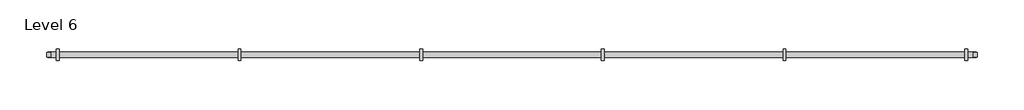
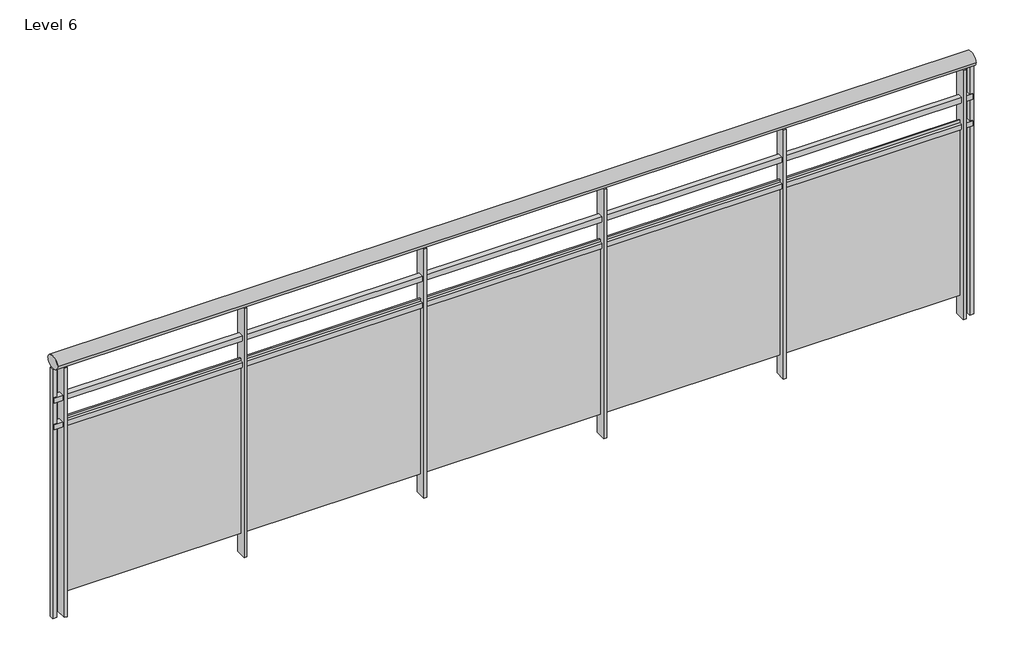
# One storey: 1 railing.
"""IFC4 building model written with IfcOpenShell, lengths in millimetres."""

from ifc_helpers import new_model, si_unit, point, frame, origin, place, context, project, spatial, polyline, ellipse_curve, trimmed, outline, extrude, element, save
from ifc_brep_helpers import plane_surface, extruded_surface, advanced_brep

model = new_model("IFC4")

# Units and contexts
model_context = context("Model", 3, world=origin())
ifc_project = project(units=[si_unit("LENGTHUNIT", "METRE", prefix="MILLI")], contexts=[model_context])

# Site, building, storey
site = spatial("IfcSite", under=ifc_project)
building = spatial("IfcBuilding", under=site)
storey = spatial("IfcBuildingStorey", under=building, Name="Level 6", Elevation=16002.0)

# Railing
placement = place(None, origin())
element("IfcRailing", 1, ObjectType="Glass Panel - Bottom Fill", at=placement, inside=storey, context=model_context, shape_type="SolidModel", body=[
    advanced_brep(
    [(-5729.1673724, -5829.5544725, 17221.2), (-5729.1673724, -5905.7544725, 17221.2), (-1576.8982041, -5829.5544725, 17221.2), (-1576.8982041, -5905.7544725, 17221.2)],
    [
        (0, 1, ellipse_curve(frame((-5729.1673724, -5867.6544725, 17221.2), z_axis=(-1.0, 0.0, 0.0), x_axis=(0.0, -1.0, 0.0)), 38.1, 28.575)),
        (1, 0, ellipse_curve(frame((-5729.1673724, -5867.6544725, 17221.2), z_axis=(-1.0, 0.0, 0.0), x_axis=(0.0, -1.0, 0.0)), 38.1, 28.575)),
        (2, 3, ellipse_curve(frame((-1576.8982041, -5867.6544725, 17221.2), z_axis=(1.0, 0.0, 0.0), x_axis=(0.0, -1.0, 0.0)), 38.1, 28.575)),
        (3, 2, ellipse_curve(frame((-1576.8982041, -5867.6544725, 17221.2), z_axis=(1.0, 0.0, 0.0), x_axis=(0.0, -1.0, 0.0)), 38.1, 28.575)),
        (0, 2),
        (3, 1),
    ],
    [
        plane_surface(frame((-5729.1673724, -5867.6544725, 17221.2), z_axis=(-1.0, 0.0, 0.0), x_axis=(0.0, 1.0, 0.0))),
        plane_surface(frame((-1576.8982041, -5867.6544725, 17221.2), z_axis=(1.0, 0.0, 0.0), x_axis=(0.0, 1.0, 0.0))),
        extruded_surface(trimmed(ellipse_curve(frame((-1576.8982041, -5867.6544725, 17221.2), z_axis=(-1.0, 0.0, 0.0), x_axis=(0.0, -1.0, 0.0)), 38.1, 28.575), [point((-1576.8982041, -5829.5544725, 17221.2))], [point((-1576.8982041, -5905.7544725, 17221.2))], True, "CARTESIAN"), (-4152.2691683, 0.0, 0.0), 4152.2691683),
        extruded_surface(trimmed(ellipse_curve(frame((-1576.8982041, -5867.6544725, 17221.2), z_axis=(-1.0, 0.0, 0.0), x_axis=(0.0, -1.0, 0.0)), 38.1, 28.575), [point((-1576.8982041, -5905.7544725, 17221.2))], [point((-1576.8982041, -5829.5544725, 17221.2))], True, "CARTESIAN"), (-4152.2691683, 0.0, 0.0), 4152.2691683),
    ],
    [
        (0, [[1, 2]]),
        (1, [[3, 4]]),
        (2, [[-1, 5, -4, 6]]),
        (3, [[-2, -6, -3, -5]]),
    ],
),
    extrude(outline(polyline([(-5729.1673724, -5880.3544725), (-5729.1673724, -5854.9544725), (-1576.8982041, -5854.9544725), (-1576.8982041, -5880.3544725), (-5729.1673724, -5880.3544725)])), frame((0.0, 0.0, 17030.7), z_axis=(0.0, 0.0, 1.0), x_axis=(1.0, 0.0, 0.0)), (0.0, 0.0, 1.0), 25.4),
    extrude(outline(polyline([(-5729.1673724, -5880.3544725), (-5729.1673724, -5854.9544725), (-1576.8982041, -5854.9544725), (-1576.8982041, -5880.3544725), (-5729.1673724, -5880.3544725)])), frame((0.0, 0.0, 16903.7), z_axis=(0.0, 0.0, 1.0), x_axis=(1.0, 0.0, 0.0)), (0.0, 0.0, 1.0), 25.4),
    extrude(outline(polyline([(-1627.3827882, -5893.0544725), (-1627.3827882, -5842.2544725), (-1614.6827882, -5842.2544725), (-1614.6827882, -5893.0544725), (-1627.3827882, -5893.0544725)])), frame((0.0, 0.0, 16002.0), z_axis=(0.0, 0.0, 1.0), x_axis=(1.0, 0.0, 0.0)), (0.0, 0.0, 1.0), 1190.625),
    extrude(outline(polyline([(-2433.8327882, -5861.1193155), (-1621.0327882, -5861.1193155), (-1621.0327882, -5867.4693155), (-2433.8327882, -5867.4693155), (-2433.8327882, -5861.1193155)])), frame((0.0, 0.0, 16103.6), z_axis=(0.0, 0.0, 1.0), x_axis=(1.0, 0.0, 0.0)), (0.0, 0.0, 1.0), 838.2),
    extrude(outline(polyline([(-2440.1827882, -5893.0544725), (-2440.1827882, -5842.2544725), (-2427.4827882, -5842.2544725), (-2427.4827882, -5893.0544725), (-2440.1827882, -5893.0544725)])), frame((0.0, 0.0, 16002.0), z_axis=(0.0, 0.0, 1.0), x_axis=(1.0, 0.0, 0.0)), (0.0, 0.0, 1.0), 1190.625),
    extrude(outline(polyline([(-3246.6327882, -5861.1193155), (-2433.8327882, -5861.1193155), (-2433.8327882, -5867.4693155), (-3246.6327882, -5867.4693155), (-3246.6327882, -5861.1193155)])), frame((0.0, 0.0, 16103.6), z_axis=(0.0, 0.0, 1.0), x_axis=(1.0, 0.0, 0.0)), (0.0, 0.0, 1.0), 838.2),
    extrude(outline(polyline([(-3252.9827882, -5893.0544725), (-3252.9827882, -5842.2544725), (-3240.2827882, -5842.2544725), (-3240.2827882, -5893.0544725), (-3252.9827882, -5893.0544725)])), frame((0.0, 0.0, 16002.0), z_axis=(0.0, 0.0, 1.0), x_axis=(1.0, 0.0, 0.0)), (0.0, 0.0, 1.0), 1190.625),
    extrude(outline(polyline([(-4059.4327882, -5861.1193155), (-3246.6327882, -5861.1193155), (-3246.6327882, -5867.4693155), (-4059.4327882, -5867.4693155), (-4059.4327882, -5861.1193155)])), frame((0.0, 0.0, 16103.6), z_axis=(0.0, 0.0, 1.0), x_axis=(1.0, 0.0, 0.0)), (0.0, 0.0, 1.0), 838.2),
    extrude(outline(polyline([(-4065.7827882, -5893.0544725), (-4065.7827882, -5842.2544725), (-4053.0827882, -5842.2544725), (-4053.0827882, -5893.0544725), (-4065.7827882, -5893.0544725)])), frame((0.0, 0.0, 16002.0), z_axis=(0.0, 0.0, 1.0), x_axis=(1.0, 0.0, 0.0)), (0.0, 0.0, 1.0), 1190.625),
    extrude(outline(polyline([(-4872.2327882, -5861.1193155), (-4059.4327882, -5861.1193155), (-4059.4327882, -5867.4693155), (-4872.2327882, -5867.4693155), (-4872.2327882, -5861.1193155)])), frame((0.0, 0.0, 16103.6), z_axis=(0.0, 0.0, 1.0), x_axis=(1.0, 0.0, 0.0)), (0.0, 0.0, 1.0), 838.2),
    extrude(outline(polyline([(-4878.5827882, -5893.0544725), (-4878.5827882, -5842.2544725), (-4865.8827882, -5842.2544725), (-4865.8827882, -5893.0544725), (-4878.5827882, -5893.0544725)])), frame((0.0, 0.0, 16002.0), z_axis=(0.0, 0.0, 1.0), x_axis=(1.0, 0.0, 0.0)), (0.0, 0.0, 1.0), 1190.625),
    extrude(outline(polyline([(-5685.0327882, -5861.1193155), (-4872.2327882, -5861.1193155), (-4872.2327882, -5867.4693155), (-5685.0327882, -5867.4693155), (-5685.0327882, -5861.1193155)])), frame((0.0, 0.0, 16103.6), z_axis=(0.0, 0.0, 1.0), x_axis=(1.0, 0.0, 0.0)), (0.0, 0.0, 1.0), 838.2),
    extrude(outline(polyline([(-5691.3827882, -5893.0544725), (-5691.3827882, -5842.2544725), (-5678.6827882, -5842.2544725), (-5678.6827882, -5893.0544725), (-5691.3827882, -5893.0544725)])), frame((0.0, 0.0, 16002.0), z_axis=(0.0, 0.0, 1.0), x_axis=(1.0, 0.0, 0.0)), (0.0, 0.0, 1.0), 1190.625),
    extrude(outline(polyline([(-1589.5982041, -5877.1794725), (-1589.5982041, -5858.1294725), (-1570.5482041, -5858.1294725), (-1570.5482041, -5877.1794725), (-1589.5982041, -5877.1794725)])), frame((0.0, 0.0, 16002.0), z_axis=(0.0, 0.0, 1.0), x_axis=(1.0, 0.0, 0.0)), (0.0, 0.0, 1.0), 1190.625),
    extrude(outline(polyline([(-5735.5173724, -5877.1794725), (-5735.5173724, -5858.1294725), (-5716.4673724, -5858.1294725), (-5716.4673724, -5877.1794725), (-5735.5173724, -5877.1794725)])), frame((0.0, 0.0, 16002.0), z_axis=(0.0, 0.0, 1.0), x_axis=(1.0, 0.0, 0.0)), (0.0, 0.0, 1.0), 1190.625),
])

save(model, "model.ifc")

# Revit data of these elements
# Type "Glass Panel - Bottom Fill"
#   Assembly Code = "C2010400"
#   built-in parameter 1008612 = 0.0416667 (stored number, unit not read)
#   built-in parameter 1008611 = 0.0416667 (stored number, unit not read)
#   built-in parameter 1008609 = 0.333333 (stored number, unit not read)
#   built-in parameter 1008604 = 0.166667 (stored number, unit not read)
#   built-in parameter 1008603 = 0.166667 (stored number, unit not read)
#   Railing Height = 4' - 0"
#   built-in parameter 1008630 = 2
#   built-in parameter 1008610 = 2
#   built-in parameter 1008618 = Baluster - Square : 3/4"
# Element 1 (IfcRailing, "Glass Panel - Bottom Fill")
#   Phase Created = New Construction
#   Materials on its faces: "Glass"
# Materials
#   "Glass": class "Glass", colour RGB 0 128 192, transparency 0.75, Description = "Soda Lime Glass", Cost = 0
